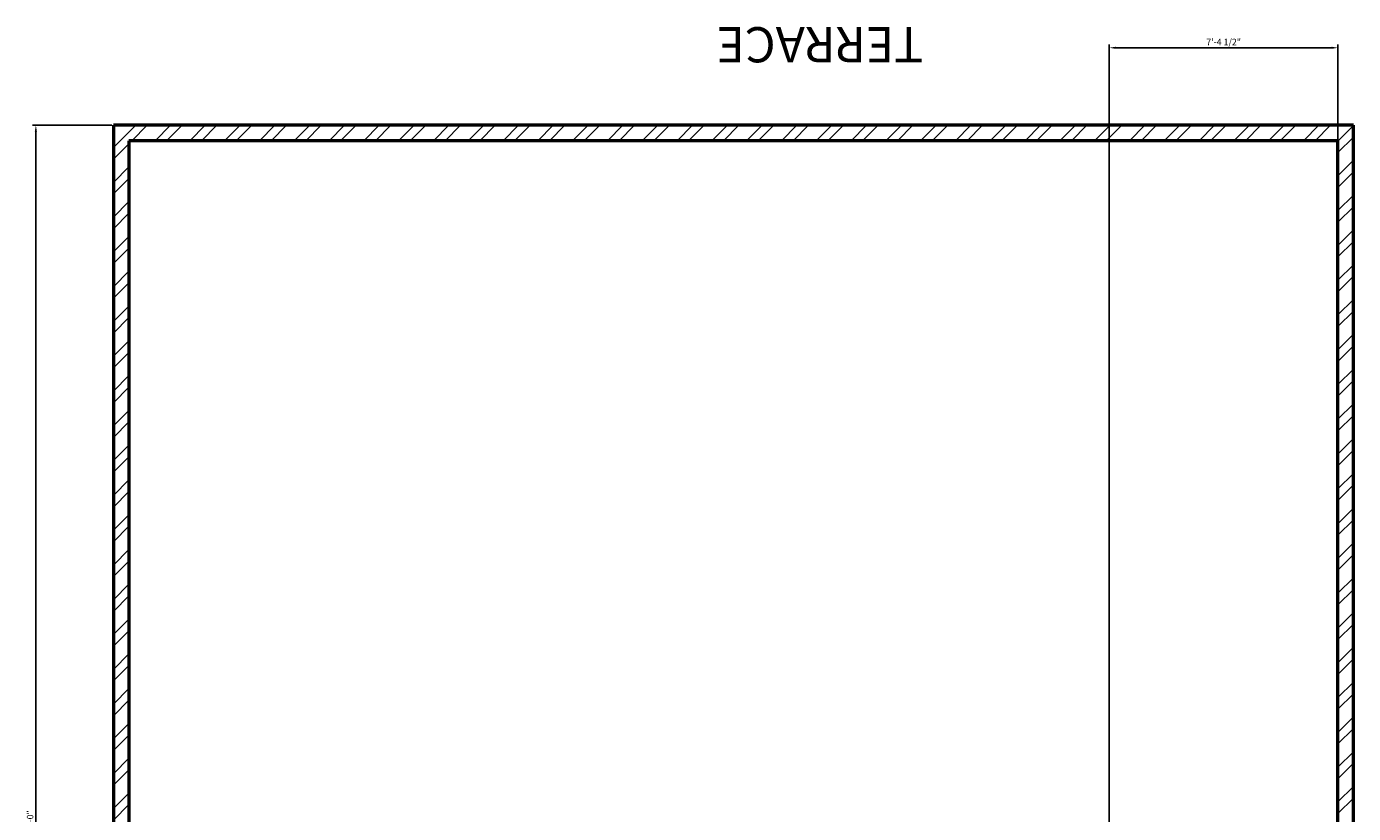
# Model space of a CAD drawing. Units: inches. Extents: x 244 to 2800, y 1060 to 1700.
# Tile 2 of 13: x 244 to 757, y 1366 to 1671. Entities that reach past the tile are written whole.
import ezdxf

# ---------------------------------------------------------------- set-up
doc = ezdxf.new("R2010")
doc.units = ezdxf.units.IN
for name, color, linetype, lineweight in [('A-ANNO-DIMS', 2, 'Continuous', 18), ('A-ANNO-TEXT', 1, 'Continuous', 18), ('A-WALL', 7, 'Continuous', 50), ('A-WALL-PATT', 8, 'Continuous', 13)]:
    doc.layers.add(name, color=color, linetype=linetype, lineweight=lineweight)
doc.styles.get("Standard").update_dxf_attribs({"font": 'arial.ttf'})
doc.dimstyles.new('ISO-25', dxfattribs={"dimtxt": 2.5, "dimasz": 2.5, "dimexe": 1.25, "dimexo": 0.625, "dimtad": 1, "dimlunit": 4, "dimtxsty": 'Standard', "dimcen": 2.5, "dimadec": 0, "dimazin": 0, "dimtfac": 1, "dimtmove": 0, "dimatfit": 3, "dimfxl": 1, "dimarcsym": 0})

# ---------------------------------------------------------------- blocks, each defined once
blk = doc.blocks.new('*D157')
at = {"layer": 'A-ANNO-DIMS', "color": 0, "lineweight": -2, "transparency": 16777216}
for p, q in [((276.67, 1632.99), (246.05, 1632.99)), ((247.3, 1095.49), (247.3, 1630.49)), ((276.67, 1092.99), (246.05, 1092.99))]:
    blk.add_line(p, q, dxfattribs=at)
at = {"layer": 'A-ANNO-DIMS', "color": 0, "transparency": 16777216}
for points in [[(246.88, 1630.49), (247.71, 1630.49), (247.3, 1632.99)], [(246.88, 1095.49), (247.71, 1095.49), (247.3, 1092.99)]]:
    blk.add_solid(points, dxfattribs=at)
at = {"layer": 'Defpoints', "color": 0, "transparency": 16777216}
for p in [(247.3, 1632.99), (277.3, 1632.99), (277.3, 1092.99)]:
    blk.add_point(p, dxfattribs=at)
at = {"layer": 'A-ANNO-DIMS', "color": 0, "transparency": 16777216, "insert": (245.39, 1362.99), "char_height": 2.5, "attachment_point": 5, "rotation": 90}
blk.add_mtext('45\'-0"', dxfattribs=at)
blk = doc.blocks.new('*D158')
at = {"layer": 'A-ANNO-DIMS', "color": 0, "lineweight": -2, "transparency": 16777216}
for p, q in [((662.8, 1243.61), (662.8, 1664.24)), ((751.3, 1243.61), (751.3, 1664.24)), ((665.3, 1662.99), (748.8, 1662.99))]:
    blk.add_line(p, q, dxfattribs=at)
at = {"layer": 'A-ANNO-DIMS', "color": 0, "transparency": 16777216}
for points in [[(665.3, 1663.4), (665.3, 1662.57), (662.8, 1662.99)], [(748.8, 1663.4), (748.8, 1662.57), (751.3, 1662.99)]]:
    blk.add_solid(points, dxfattribs=at)
at = {"layer": 'Defpoints', "color": 0, "transparency": 16777216}
for p in [(751.3, 1662.99), (662.8, 1242.99), (751.3, 1242.99)]:
    blk.add_point(p, dxfattribs=at)
at = {"layer": 'A-ANNO-DIMS', "color": 0, "transparency": 16777216, "insert": (707.05, 1664.9), "char_height": 2.5, "attachment_point": 5}
blk.add_mtext('7\'-4 1/2"', dxfattribs=at)

msp = doc.modelspace()

# ---------------------------------------------------------------- hatches: boundary and pattern name
at = {"layer": 'A-WALL-PATT'}
h = msp.add_hatch(dxfattribs=at)
h.set_pattern_fill('ANSI32', color=256)
h.paths.add_polyline_path([(757.295, 1632.986), (277.295, 1632.986), (277.295, 1092.986), (757.295, 1092.986)])
h.paths.add_polyline_path([(283.295, 1098.986), (283.295, 1626.986), (751.295, 1626.986), (751.295, 1098.986), (667.295, 1098.986)], flags=16)
h.paths.add_polyline_path([(667.295, 1242.986), (703.295, 1242.986), (703.295, 1134.986), (715.295, 1134.986), (715.295, 1242.986), (751.295, 1242.986), (751.295, 1134.986), (667.295, 1134.986)], flags=0)

# ---------------------------------------------------------------- linework, layer by layer
at = {"layer": 'A-WALL'}
for p, q in [((757.295, 1632.986), (277.295, 1632.986)), ((277.295, 1632.986), (277.295, 1092.986)), ((757.295, 1092.986), (757.295, 1632.986)), ((751.295, 1626.986), (283.295, 1626.986)), ((283.295, 1626.986), (283.295, 1098.986)), ((751.295, 1098.986), (751.295, 1626.986))]:
    msp.add_line(p, q, dxfattribs=at)

# ---------------------------------------------------------------- texts
at = {"layer": 'A-ANNO-TEXT', "insert": (590.737, 1657.323), "char_height": 13.6485, "attachment_point": 1, "rotation": 180}
msp.add_mtext_dynamic_manual_height_columns('TERRACE', width=25.27039, gutter_width=68.243, heights=[0], dxfattribs=at)

# ---------------------------------------------------------------- dimensions: what is measured, and where the dimension line sits
at = {"layer": 'A-ANNO-DIMS'}
dim = msp.add_linear_dim(base=(751.295, 1662.986), p1=(662.795, 1242.986), p2=(751.295, 1242.986), dimstyle='ISO-25', override={"dimdec": 1, "dimlfac": 1, "dimrnd": 0, "dimzin": 1, "dimdsep": 46, "dimlunit": 4, "dimfrac": 2}, dxfattribs=at)
dim.commit()
dim.dimension.update_dxf_attribs({"geometry": '*D158', "text_midpoint": (707.045, 1664.904)})
dim = msp.add_linear_dim(base=(247.295, 1632.986), p1=(277.295, 1092.986), p2=(277.295, 1632.986), angle=90, dimstyle='ISO-25', override={"dimdec": 1, "dimlfac": 1, "dimrnd": 0, "dimzin": 1, "dimdsep": 46, "dimlunit": 4, "dimfrac": 2}, dxfattribs=at)
dim.commit()
dim.dimension.update_dxf_attribs({"geometry": '*D157', "text_midpoint": (245.394, 1362.986)})

doc.saveas('drawing.dxf')
